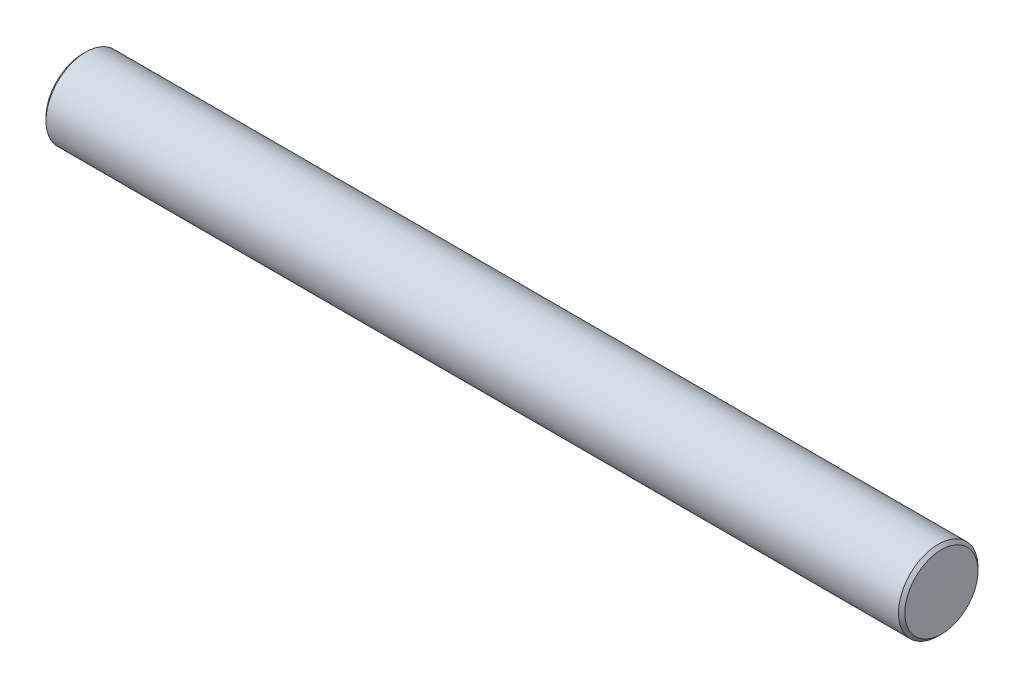
SolidWorks part; units mm, degrees
material "Plain Carbon Steel"
ref_plane "Front Plane" through (0, 0, 0) normal (0, 0, 1) x (1, 0, 0)
ref_plane "Top Plane" through (0, 0, 0) normal (0, 1, 0) x (1, 0, 0)
ref_plane "Right Plane" through (0, 0, 0) normal (1, 0, 0) x (0, 0, -1)
sketch "Shaft Half Profile" plane through (0, 0, 0) normal (0, 0, 1) x (1, 0, 0)
  line L0 (-270, 0) -> (270, 0)
  line L1 (270, 25) -> (-270, 25)
  line L2 (270, 25) -> (270, 0)
  line L4 (-270, 25) -> (-270, 0)
  line L5 (270, 25) -> (0, 0) construction
  line L6 (0, 0) -> (-270, 25) construction
  point P0 (0, 0)
  dimension "D1" = 25
  dimension "540" = 540
revolve "Shaft Ø50x540" add sketch "Shaft Half Profile" angle 360 about L0
chamfer "End Chamfers 2x45°" distance 2 angle 45 2 edges at (-270, -25, 0) (270, -25, 0)
